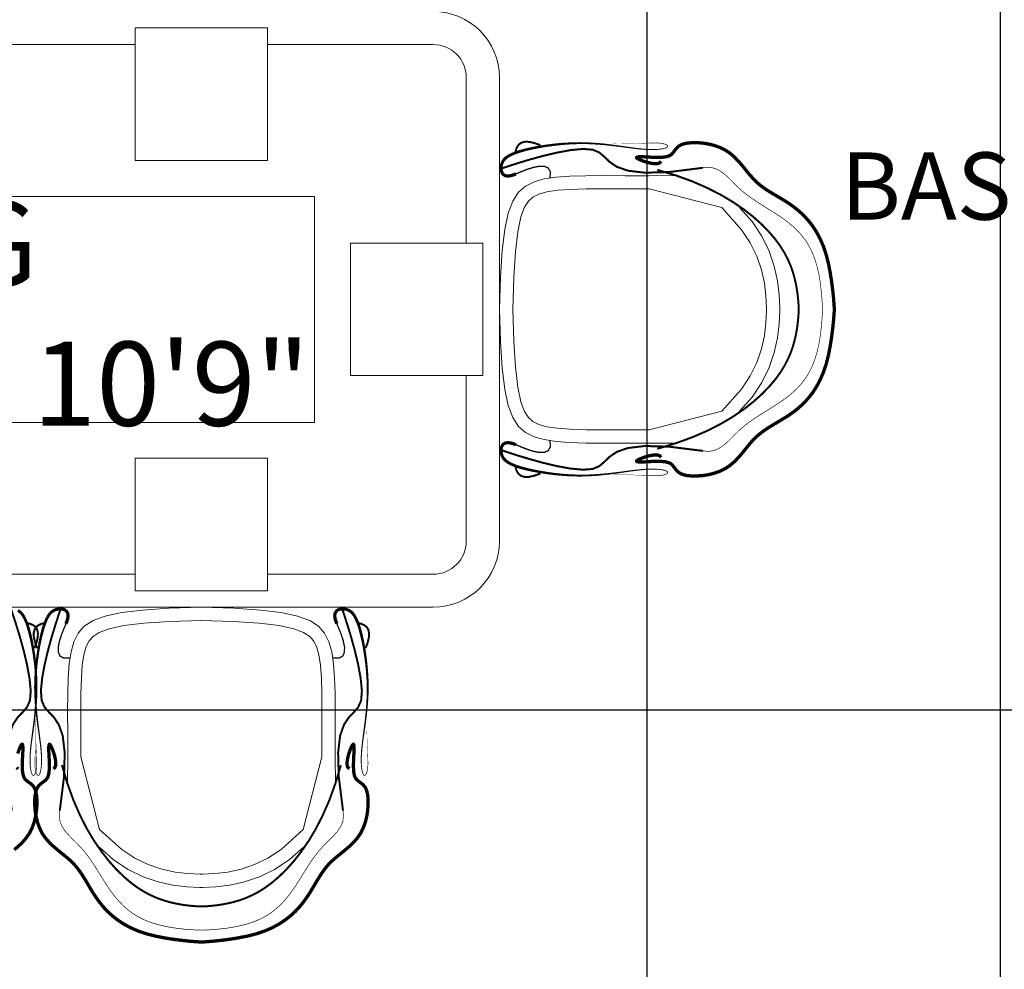
# Model space of a CAD drawing. Units: inches. Extents: x 870 to 1431, y 383 to 1070.
# Tile 6 of 9: x 1171 to 1230, y 661 to 718. Entities that reach past the tile are written whole.
import ezdxf

# ---------------------------------------------------------------- set-up
doc = ezdxf.new("R2010")
doc.units = ezdxf.units.IN
doc.header["$MEASUREMENT"] = 0
for name, color, linetype, lineweight in [('A-ANNO-DIMS', 2, 'Continuous', 18), ('A-AREA-IDEN', 7, 'Continuous', 25), ('A-FURN', 8, 'Continuous', 18)]:
    doc.layers.add(name, color=color, linetype=linetype, lineweight=lineweight)
doc.styles.get("Standard").update_dxf_attribs({"font": 'arial.ttf'})
doc.dimstyles.get("Standard").update_dxf_attribs({"dimtxt": 4, "dimasz": 0.18, "dimexe": 0.18, "dimexo": 0.0625, "dimgap": 0.09, "dimtad": 0, "dimtih": 1, "dimtoh": 1, "dimdec": 0, "dimrnd": 6, "dimzin": 0, "dimdsep": 46, "dimlunit": 3, "dimtxsty": 'Standard', "dimcen": 0.09, "dimadec": 0, "dimazin": 0, "dimtfac": 1, "dimtdec": 0, "dimtofl": 0, "dimtmove": 0, "dimatfit": 3, "dimfxl": 1, "dimtolj": 1, "dimtzin": 0, "dimarcsym": 0})

# ---------------------------------------------------------------- blocks, each defined once
blk = doc.blocks.new('ОГ53_на8персон_стол1900х900')
for p, q in [((400, 254.3), (400, 54.3)), ((600, 254.3), (400, 254.3)), ((600, 54.3), (600, 254.3)), ((100, 229.3), (400, 229.3)), ((600, 229.3), (850, 229.3)), ((900, 179.3), (900, -70.7)), ((950, 179.3), (950, -520.7)), ((400, 54.3), (600, 54.3)), ((670.7, 0), (-670.7, 0)), ((670.7, -341.4), (670.7, 0)), ((725, -270.7), (725, -70.7)), ((725, -70.7), (925, -70.7)), ((925, -70.7), (925, -270.7)), ((925, -270.7), (725, -270.7)), ((900, -270.7), (900, -520.7)), ((-670.7, -341.4), (670.7, -341.4)), ((400, -595.7), (400, -395.7)), ((400, -395.7), (600, -395.7)), ((600, -395.7), (600, -595.7)), ((400, -570.7), (100, -570.7)), ((850, -570.7), (600, -570.7)), ((600, -595.7), (400, -595.7)), ((850, -620.7), (-850, -620.7))]:
    blk.add_line(p, q)
for points in [[(974.9, 33.8, 5, 4.91, 0), (968.1, 31.4, 4.91, 4.84, 0), (962.8, 30.6, 4.84, 4.78, 0), (958.7, 31.2, 4.78, 4.74, 0), (955.8, 33, 4.74, 4.7, 0), (953.9, 35.6, 4.7, 4.65, 0), (952.9, 38.8, 4.65, 4.61, 0), (952.5, 42.3, 4.61, 4.56, 0), (952.8, 45.8, 4.56, 4.52, 0), (953.5, 49.1, 4.52, 4.47, 0), (954.8, 52.2, 4.47, 4.43, 0), (956.7, 55.2, 4.43, 4.38, 0), (959.5, 58, 4.38, 4.32, 0), (963.2, 60.6, 4.32, 4.25, 0), (967.9, 63.2, 4.25, 4.17, 0), (973.8, 65.6, 4.17, 4.07, 0), (981, 68, 4.07, 3.95, 0), (989.6, 70.4, 3.95, 3.82, 0), (999.3, 72.6, 3.82, 3.68, 0), (1010.1, 74.7, 3.68, 3.53, 0), (1021.6, 76.5, 3.53, 3.37, 0), (1033.7, 78.1, 3.37, 3.21, 0), (1046.2, 79.3, 3.21, 3.05, 0), (1058.8, 80.1, 3.05, 2.88, 0), (1071.4, 80.4, 2.88, 2.72, 0), (1083.8, 80.2, 2.72, 2.57, 0), (1095.8, 79.5, 2.57, 2.41, 0), (1107.4, 78.6, 2.41, 2.27, 0), (1118.5, 77.3, 2.27, 2.13, 0), (1129, 76, 2.13, 2, 0), (1138.9, 74.6, 2, 1.88, 0), (1148, 73.4, 1.88, 1.78, 0), (1156.3, 72.3, 1.78, 1.68, 0), (1163.7, 71.5, 1.68, 1.59, 0), (1170.3, 71, 1.59, 1.52, 0), (1176.1, 70.7, 1.52, 1.45, 0), (1181.2, 70.7, 1.45, 1.4, 0), (1185.6, 70.7, 1.4, 1.35, 0), (1189.4, 71, 1.35, 1.3, 0), (1192.6, 71.3, 1.3, 1.27, 0), (1195.3, 71.7, 1.27, 1.24, 0), (1197.6, 72.1, 1.24, 1.21, 0), (1199.5, 72.6, 1.21, 1.19, 0), (1201, 73.1, 1.19, 1.18, 0), (1202.2, 73.6, 1.18, 1.16, 0), (1203, 74.1, 1.16, 1.15, 0), (1203.6, 74.6, 1.15, 1.14, 0), (1203.9, 75.1, 1.14, 1.14, 0), (1204, 75.6, 1.14, 1.13, 0), (1203.9, 76.2, 1.13, 1.12, 0), (1203.6, 76.6, 1.12, 1.12, 0), (1203.2, 77.1, 1.12, 1.11, 0), (1202.6, 77.6, 1.11, 1.09, 0), (1201.8, 78, 1.09, 1.08, 0), (1200.9, 78.4, 1.08, 1.07, 0), (1199.8, 78.9, 1.07, 1.05, 0), (1198.6, 79.2, 1.05, 1.03, 0), (1197.2, 79.6, 1.03, 1.01, 0), (1195.6, 79.9, 1.01, 0.986, 0), (1193.8, 80.2, 0.986, 0.959, 0), (1191.7, 80.4, 0.959, 0.926, 0), (1189.2, 80.6, 0.926, 0.889, 0), (1186.3, 80.7, 0.889, 0.846, 0), (1183, 80.7, 0.846, 0.796, 0), (1179.1, 80.6, 0.796, 0.738, 0), (1174.7, 80.4, 0.738, 0.672, 0), (1169.6, 80.2, 0.672, 0.595, 0), (1163.7, 79.9, 0.595, 0.506, 0), (1156.8, 79.6, 0.506, 0.404, 0), (1148.9, 79.4, 0.404, 0.286, 0), (1139.9, 79.2, 0.286, 0.152, 0), (1129.5, 79.2, 0.152, 0, 0), (1117.8, 79.4, 0, 0, 0)], [(974.9, -375.1, 5, 4.91, 0), (968.1, -372.7, 4.91, 4.84, 0), (962.8, -372, 4.84, 4.78, 0), (958.7, -372.6, 4.78, 4.74, 0), (955.8, -374.3, 4.74, 4.7, 0), (953.9, -376.9, 4.7, 4.65, 0), (952.9, -380.1, 4.65, 4.61, 0), (952.5, -383.6, 4.61, 4.56, 0), (952.8, -387.1, 4.56, 4.52, 0), (953.5, -390.5, 4.52, 4.47, 0), (954.8, -393.6, 4.47, 4.43, 0), (956.7, -396.6, 4.43, 4.38, 0), (959.5, -399.3, 4.38, 4.32, 0), (963.2, -402, 4.32, 4.25, 0), (967.9, -404.5, 4.25, 4.17, 0), (973.8, -407, 4.17, 4.07, 0), (981, -409.4, 4.07, 3.95, 0), (989.6, -411.7, 3.95, 3.82, 0), (999.3, -414, 3.82, 3.68, 0), (1010.1, -416, 3.68, 3.53, 0), (1021.6, -417.9, 3.53, 3.37, 0), (1033.7, -419.5, 3.37, 3.21, 0), (1046.2, -420.7, 3.21, 3.05, 0), (1058.8, -421.5, 3.05, 2.88, 0), (1071.4, -421.8, 2.88, 2.72, 0), (1083.8, -421.6, 2.72, 2.57, 0), (1095.8, -420.9, 2.57, 2.41, 0), (1107.4, -419.9, 2.41, 2.27, 0), (1118.5, -418.7, 2.27, 2.13, 0), (1129, -417.4, 2.13, 2, 0), (1138.9, -416, 2, 1.88, 0), (1148, -414.7, 1.88, 1.78, 0), (1156.3, -413.7, 1.78, 1.68, 0), (1163.7, -412.9, 1.68, 1.59, 0), (1170.3, -412.4, 1.59, 1.52, 0), (1176.1, -412.1, 1.52, 1.45, 0), (1181.2, -412, 1.45, 1.4, 0), (1185.6, -412.1, 1.4, 1.35, 0), (1189.4, -412.3, 1.35, 1.3, 0), (1192.6, -412.7, 1.3, 1.27, 0), (1195.3, -413, 1.27, 1.24, 0), (1197.6, -413.5, 1.24, 1.21, 0), (1199.5, -413.9, 1.21, 1.19, 0), (1201, -414.4, 1.19, 1.18, 0), (1202.2, -414.9, 1.18, 1.16, 0), (1203, -415.4, 1.16, 1.15, 0), (1203.6, -416, 1.15, 1.14, 0), (1203.9, -416.5, 1.14, 1.14, 0), (1204, -417, 1.14, 1.13, 0), (1203.9, -417.5, 1.13, 1.12, 0), (1203.6, -418, 1.12, 1.12, 0), (1203.2, -418.5, 1.12, 1.11, 0), (1202.6, -418.9, 1.11, 1.09, 0), (1201.8, -419.4, 1.09, 1.08, 0), (1200.9, -419.8, 1.08, 1.07, 0), (1199.8, -420.2, 1.07, 1.05, 0), (1198.6, -420.6, 1.05, 1.03, 0), (1197.2, -421, 1.03, 1.01, 0), (1195.6, -421.3, 1.01, 0.986, 0), (1193.8, -421.6, 0.986, 0.959, 0), (1191.7, -421.8, 0.959, 0.926, 0), (1189.2, -422, 0.926, 0.889, 0), (1186.3, -422, 0.889, 0.846, 0), (1183, -422, 0.846, 0.796, 0), (1179.1, -422, 0.796, 0.738, 0), (1174.7, -421.8, 0.738, 0.672, 0), (1169.6, -421.5, 0.672, 0.595, 0), (1163.7, -421.2, 0.595, 0.506, 0), (1156.8, -421, 0.506, 0.404, 0), (1148.9, -420.7, 0.404, 0.286, 0), (1139.9, -420.6, 0.286, 0.152, 0), (1129.5, -420.6, 0.152, 0, 0), (1117.8, -420.7, 0, 0, 0)], [(222.9, -625.5, 4.47, 4.43, 0), (225.9, -627.4, 4.43, 4.38, 0), (228.7, -630.2, 4.38, 4.32, 0), (231.3, -633.9, 4.32, 4.25, 0), (233.8, -638.6, 4.25, 4.17, 0), (236.3, -644.5, 4.17, 4.07, 0), (238.7, -651.7, 4.07, 3.95, 0), (241, -660.3, 3.95, 3.82, 0), (243.3, -670, 3.82, 3.68, 0), (245.4, -680.8, 3.68, 3.53, 0), (247.2, -692.3, 3.53, 3.37, 0), (248.8, -704.4, 3.37, 3.21, 0), (250, -716.9, 3.21, 3.05, 0), (250.8, -729.5, 3.05, 2.88, 0), (251.1, -742.1, 2.88, 2.72, 0), (250.9, -754.5, 2.72, 2.57, 0), (250.2, -766.5, 2.57, 2.41, 0), (249.2, -778.1, 2.41, 2.27, 0), (248, -789.2, 2.27, 2.13, 0), (246.7, -799.7, 2.13, 2, 0), (245.3, -809.6, 2, 1.88, 0), (244.1, -818.7, 1.88, 1.78, 0), (243, -827, 1.78, 1.68, 0), (242.2, -834.4, 1.68, 1.59, 0), (241.7, -841, 1.59, 1.52, 0), (241.4, -846.8, 1.52, 1.45, 0), (241.3, -851.9, 1.45, 1.4, 0), (241.4, -856.3, 1.4, 1.35, 0), (241.6, -860.1, 1.35, 1.3, 0), (242, -863.3, 1.3, 1.27, 0), (242.4, -866, 1.27, 1.24, 0), (242.8, -868.3, 1.24, 1.21, 0), (243.3, -870.2, 1.21, 1.19, 0), (243.8, -871.7, 1.19, 1.18, 0), (244.3, -872.9, 1.18, 1.16, 0), (244.8, -873.7, 1.16, 1.15, 0), (245.3, -874.3, 1.15, 1.14, 0), (245.8, -874.6, 1.14, 1.14, 0), (246.3, -874.7, 1.14, 1.13, 0), (246.8, -874.6, 1.13, 1.12, 0), (247.3, -874.3, 1.12, 1.12, 0), (247.8, -873.9, 1.12, 1.11, 0), (248.3, -873.3, 1.11, 1.09, 0), (248.7, -872.5, 1.09, 1.08, 0), (249.1, -871.6, 1.08, 1.07, 0), (249.5, -870.5, 1.07, 1.05, 0), (249.9, -869.2, 1.05, 1.03, 0), (250.3, -867.9, 1.03, 1.01, 0), (250.6, -866.3, 1.01, 0.986, 0), (250.9, -864.5, 0.986, 0.959, 0), (251.1, -862.4, 0.959, 0.926, 0), (251.3, -859.9, 0.926, 0.889, 0), (251.4, -857, 0.889, 0.846, 0), (251.4, -853.7, 0.846, 0.796, 0), (251.3, -849.8, 0.796, 0.738, 0), (251.1, -845.4, 0.738, 0.672, 0), (250.8, -840.3, 0.672, 0.595, 0), (250.6, -834.3, 0.595, 0.506, 0), (250.3, -827.5, 0.506, 0.404, 0), (250.1, -819.6, 0.404, 0.286, 0), (249.9, -810.5, 0.286, 0.152, 0), (249.9, -800.2, 0.152, 0, 0), (250, -788.5, 0, 0, 0)], [(295.5, -645.6, 5, 4.91, 0), (298, -638.8, 4.91, 4.84, 0), (298.7, -633.5, 4.84, 4.78, 0), (298.1, -629.4, 4.78, 4.74, 0), (296.3, -626.5, 4.74, 4.7, 0), (293.7, -624.6, 4.7, 4.65, 0), (290.6, -623.5, 4.65, 4.61, 0), (287.1, -623.2, 4.61, 4.56, 0), (283.5, -623.5, 4.56, 4.52, 0), (280.2, -624.2, 4.52, 4.47, 0), (277.1, -625.5, 4.47, 4.43, 0), (274.1, -627.4, 4.43, 4.38, 0), (271.3, -630.2, 4.38, 4.32, 0), (268.7, -633.9, 4.32, 4.25, 0), (266.2, -638.6, 4.25, 4.17, 0), (263.7, -644.5, 4.17, 4.07, 0), (261.3, -651.7, 4.07, 3.95, 0), (259, -660.3, 3.95, 3.82, 0), (256.7, -670, 3.82, 3.68, 0), (254.6, -680.8, 3.68, 3.53, 0), (252.8, -692.3, 3.53, 3.37, 0), (251.2, -704.4, 3.37, 3.21, 0), (250, -716.9, 3.21, 3.05, 0), (249.2, -729.5, 3.05, 2.88, 0), (248.9, -742.1, 2.88, 2.72, 0), (249.1, -754.5, 2.72, 2.57, 0), (249.8, -766.5, 2.57, 2.41, 0), (250.8, -778.1, 2.41, 2.27, 0), (252, -789.2, 2.27, 2.13, 0), (253.3, -799.7, 2.13, 2, 0), (254.7, -809.6, 2, 1.88, 0), (255.9, -818.7, 1.88, 1.78, 0), (257, -827, 1.78, 1.68, 0), (257.8, -834.4, 1.68, 1.59, 0), (258.3, -841, 1.59, 1.52, 0), (258.6, -846.8, 1.52, 1.45, 0), (258.7, -851.9, 1.45, 1.4, 0), (258.6, -856.3, 1.4, 1.35, 0), (258.4, -860.1, 1.35, 1.3, 0), (258, -863.3, 1.3, 1.27, 0), (257.6, -866, 1.27, 1.24, 0), (257.2, -868.3, 1.24, 1.21, 0), (256.7, -870.2, 1.21, 1.19, 0), (256.2, -871.7, 1.19, 1.18, 0), (255.7, -872.9, 1.18, 1.16, 0), (255.2, -873.7, 1.16, 1.15, 0), (254.7, -874.3, 1.15, 1.14, 0), (254.2, -874.6, 1.14, 1.14, 0), (253.7, -874.7, 1.14, 1.13, 0), (253.2, -874.6, 1.13, 1.12, 0), (252.7, -874.3, 1.12, 1.12, 0), (252.2, -873.9, 1.12, 1.11, 0), (251.7, -873.3, 1.11, 1.09, 0), (251.3, -872.5, 1.09, 1.08, 0), (250.9, -871.6, 1.08, 1.07, 0), (250.5, -870.5, 1.07, 1.05, 0), (250.1, -869.2, 1.05, 1.03, 0), (249.7, -867.9, 1.03, 1.01, 0), (249.4, -866.3, 1.01, 0.986, 0), (249.1, -864.5, 0.986, 0.959, 0), (248.9, -862.4, 0.959, 0.926, 0), (248.7, -859.9, 0.926, 0.889, 0), (248.6, -857, 0.889, 0.846, 0), (248.6, -853.7, 0.846, 0.796, 0), (248.7, -849.8, 0.796, 0.738, 0), (248.9, -845.4, 0.738, 0.672, 0), (249.2, -840.3, 0.672, 0.595, 0), (249.4, -834.3, 0.595, 0.506, 0), (249.7, -827.5, 0.506, 0.404, 0), (249.9, -819.6, 0.404, 0.286, 0), (250.1, -810.5, 0.286, 0.152, 0), (250.1, -800.2, 0.152, 0, 0), (250, -788.5, 0, 0, 0)], [(704.5, -645.6, 5, 4.91, 0), (702, -638.8, 4.91, 4.84, 0), (701.3, -633.5, 4.84, 4.78, 0), (701.9, -629.4, 4.78, 4.74, 0), (703.7, -626.5, 4.74, 4.7, 0), (706.3, -624.6, 4.7, 4.65, 0), (709.4, -623.5, 4.65, 4.61, 0), (712.9, -623.2, 4.61, 4.56, 0), (716.5, -623.5, 4.56, 4.52, 0), (719.8, -624.2, 4.52, 4.47, 0), (722.9, -625.5, 4.47, 4.43, 0), (725.9, -627.4, 4.43, 4.38, 0), (728.7, -630.2, 4.38, 4.32, 0), (731.3, -633.9, 4.32, 4.25, 0), (733.8, -638.6, 4.25, 4.17, 0), (736.3, -644.5, 4.17, 4.07, 0), (738.7, -651.7, 4.07, 3.95, 0), (741, -660.3, 3.95, 3.82, 0), (743.3, -670, 3.82, 3.68, 0), (745.4, -680.8, 3.68, 3.53, 0), (747.2, -692.3, 3.53, 3.37, 0), (748.8, -704.4, 3.37, 3.21, 0), (750, -716.9, 3.21, 3.05, 0), (750.8, -729.5, 3.05, 2.88, 0), (751.1, -742.1, 2.88, 2.72, 0), (750.9, -754.5, 2.72, 2.57, 0), (750.2, -766.5, 2.57, 2.41, 0), (749.2, -778.1, 2.41, 2.27, 0), (748, -789.2, 2.27, 2.13, 0), (746.7, -799.7, 2.13, 2, 0), (745.3, -809.6, 2, 1.88, 0), (744.1, -818.7, 1.88, 1.78, 0), (743, -827, 1.78, 1.68, 0), (742.2, -834.4, 1.68, 1.59, 0), (741.7, -841, 1.59, 1.52, 0), (741.4, -846.8, 1.52, 1.45, 0), (741.3, -851.9, 1.45, 1.4, 0), (741.4, -856.3, 1.4, 1.35, 0), (741.6, -860.1, 1.35, 1.3, 0), (742, -863.3, 1.3, 1.27, 0), (742.4, -866, 1.27, 1.24, 0), (742.8, -868.3, 1.24, 1.21, 0), (743.3, -870.2, 1.21, 1.19, 0), (743.8, -871.7, 1.19, 1.18, 0), (744.3, -872.9, 1.18, 1.16, 0), (744.8, -873.7, 1.16, 1.15, 0), (745.3, -874.3, 1.15, 1.14, 0), (745.8, -874.6, 1.14, 1.14, 0), (746.3, -874.7, 1.14, 1.13, 0), (746.8, -874.6, 1.13, 1.12, 0), (747.3, -874.3, 1.12, 1.12, 0), (747.8, -873.9, 1.12, 1.11, 0), (748.3, -873.3, 1.11, 1.09, 0), (748.7, -872.5, 1.09, 1.08, 0), (749.1, -871.6, 1.08, 1.07, 0), (749.5, -870.5, 1.07, 1.05, 0), (749.9, -869.2, 1.05, 1.03, 0), (750.3, -867.9, 1.03, 1.01, 0), (750.6, -866.3, 1.01, 0.986, 0), (750.9, -864.5, 0.986, 0.959, 0), (751.1, -862.4, 0.959, 0.926, 0), (751.3, -859.9, 0.926, 0.889, 0), (751.4, -857, 0.889, 0.846, 0), (751.4, -853.7, 0.846, 0.796, 0), (751.3, -849.8, 0.796, 0.738, 0), (751.1, -845.4, 0.738, 0.672, 0), (750.8, -840.3, 0.672, 0.595, 0), (750.6, -834.3, 0.595, 0.506, 0), (750.3, -827.5, 0.506, 0.404, 0), (750.1, -819.6, 0.404, 0.286, 0), (749.9, -810.5, 0.286, 0.152, 0), (749.9, -800.2, 0.152, 0, 0), (750, -788.5, 0, 0, 0)]]:
    blk.add_lwpolyline(points, format="xyseb")
for points, const_width in [([(1011.7, 77.3), (1002.5, 80.6), (994.8, 82.3), (988.5, 82.4), (983.5, 81.2), (979.7, 78.7), (976.9, 75.1), (975, 70.5), (973.8, 65)], 3), ([(1194.1, 52.8), (1192.1, 50.6), (1188.9, 49.4), (1184.9, 49.2), (1180.3, 49.7), (1175.5, 50.7), (1170.8, 52), (1166.4, 53.5), (1162.7, 55), (1159.9, 56.3), (1158, 57.4), (1157.1, 58.2), (1157.1, 58.9), (1158, 59.4), (1159.8, 59.7), (1162.5, 59.9), (1166.1, 59.8), (1170.5, 59.6), (1175.5, 59.3), (1181, 59), (1186.6, 58.9), (1192.2, 58.9), (1197.5, 59.2), (1202.2, 59.9), (1206.2, 61.1), (1209.2, 62.9), (1211.5, 65), (1213.4, 67.5), (1215.3, 70.1), (1217.4, 72.7), (1219.9, 75.2), (1223.4, 77.4), (1227.9, 79.2), (1233.8, 80.4), (1240.9, 81.1), (1248.8, 81.1), (1257.3, 80.4), (1266.1, 78.9), (1274.9, 76.7), (1283.4, 73.6), (1291.3, 69.7), (1298.4, 64.9), (1304.8, 59.3), (1310.7, 53.2), (1316.3, 46.8), (1321.6, 40.2), (1326.9, 33.7), (1332.4, 27.4), (1338.1, 21.5), (1344.4, 16.2), (1351, 11.4), (1358, 6.9), (1365.2, 2.5), (1372.6, -1.8), (1380.1, -6.3), (1387.6, -11.1), (1395, -16.4), (1402.3, -22.3), (1409.4, -29), (1416.2, -36.3), (1422.7, -44.6), (1428.7, -53.8), (1434.1, -64), (1439, -75.2), (1443.2, -87.7), (1446.7, -101.2), (1449.4, -115.3), (1451.6, -129.2), (1453.2, -142.1), (1454.4, -153.5), (1455.1, -162.5), (1455.5, -168.5), (1455.7, -170.7)], 5), ([(1257.2, 43.1), (1206.2, 36.7), (1169.4, 35.7), (1144.1, 38.7), (1127.3, 44.6), (1116.4, 51.9), (1108.5, 59.6), (1100.8, 66.2), (1090.7, 70.5), (1076, 71.6), (1057.4, 69.8), (1036.6, 66), (1015.2, 60.9), (994.5, 55.2), (976.1, 49.6), (961.6, 44.9), (952.6, 41.8)], 3), ([(974.9, 33.8), (982.7, 37.2), (991.6, 40.7), (1001, 43.6), (1010, 45.4), (1017.8, 45.4), (1023.6, 42.8), (1026.8, 37.1), (1026.4, 27.6)], 2), ([(1188.3, 40), (1216.1, 31.7), (1241.4, 22.5), (1264.2, 12.5), (1284.8, 2), (1303.1, -8.9), (1319.4, -20.1), (1333.7, -31.3), (1346.1, -42.5), (1356.8, -53.5), (1366, -64.2), (1373.7, -74.7), (1380.1, -84.9), (1385.3, -94.9), (1389.6, -104.7), (1393, -114.3), (1395.6, -123.7), (1397.7, -132.7), (1399.2, -141.4), (1400.3, -149.3), (1401, -156.4), (1401.5, -162.3), (1401.7, -166.8), (1401.8, -169.6), (1401.8, -170.7)], 3), ([(1257.2, 43.1), (1265.9, 43.9), (1273.6, 42.7), (1280.7, 39.8), (1287.3, 35.6), (1293.5, 30.4), (1299.4, 24.7), (1305.3, 18.6), (1311.3, 12.7), (1317.5, 7.2), (1323.9, 2.1), (1330.6, -2.8), (1337.4, -7.4), (1344.3, -11.8), (1351.4, -16.3), (1358.5, -20.7), (1365.7, -25.2), (1372.9, -29.9), (1380, -34.9), (1387, -40.2), (1393.8, -45.9), (1400.3, -52.2), (1406.4, -59), (1412.1, -66.5), (1417.3, -74.8), (1421.9, -83.9), (1425.9, -94), (1429.3, -105.1), (1432.2, -117.4), (1434.5, -130.9), (1436.2, -145.8), (1437.4, -162.1), (1437.8, -170.7)], 1), ([(1194.1, -394.1), (1192.1, -391.9), (1188.9, -390.8), (1184.9, -390.6), (1180.3, -391.1), (1175.5, -392), (1170.8, -393.4), (1166.4, -394.9), (1162.7, -396.3), (1159.9, -397.6), (1158, -398.7), (1157.1, -399.6), (1157.1, -400.3), (1158, -400.8), (1159.8, -401.1), (1162.5, -401.2), (1166.1, -401.2), (1170.5, -401), (1175.5, -400.7), (1181, -400.4), (1186.6, -400.2), (1192.2, -400.3), (1197.5, -400.6), (1202.2, -401.3), (1206.2, -402.5), (1209.2, -404.2), (1211.5, -406.4), (1213.4, -408.8), (1215.3, -411.4), (1217.4, -414.1), (1219.9, -416.5), (1223.4, -418.7), (1227.9, -420.5), (1233.8, -421.8), (1240.9, -422.4), (1248.8, -422.4), (1257.3, -421.7), (1266.1, -420.3), (1274.9, -418), (1283.4, -415), (1291.3, -411), (1298.4, -406.2), (1304.8, -400.7), (1310.7, -394.6), (1316.3, -388.1), (1321.6, -381.6), (1326.9, -375), (1332.4, -368.7), (1338.1, -362.9), (1344.4, -357.6), (1351, -352.8), (1358, -348.2), (1365.2, -343.9), (1372.6, -339.5), (1380.1, -335), (1387.6, -330.2), (1395, -324.9), (1402.3, -319), (1409.4, -312.4), (1416.2, -305), (1422.7, -296.8), (1428.7, -287.6), (1434.1, -277.4), (1439, -266.1), (1443.2, -253.7), (1446.7, -240.1), (1449.4, -226.1), (1451.6, -212.2), (1453.2, -199.2), (1454.4, -187.9), (1455.1, -178.9), (1455.5, -172.9), (1455.7, -170.7)], 5), ([(1188.3, -381.3), (1216.1, -373), (1241.4, -363.8), (1264.2, -353.9), (1284.8, -343.4), (1303.1, -332.5), (1319.4, -321.3), (1333.7, -310), (1346.1, -298.9), (1356.8, -287.9), (1366, -277.2), (1373.7, -266.7), (1380.1, -256.4), (1385.3, -246.4), (1389.6, -236.6), (1393, -227), (1395.6, -217.7), (1397.7, -208.6), (1399.2, -200), (1400.3, -192), (1401, -185), (1401.5, -179.1), (1401.7, -174.6), (1401.8, -171.7), (1401.8, -170.7)], 3), ([(1257.2, -384.5), (1265.9, -385.3), (1273.6, -384), (1280.7, -381.1), (1287.3, -376.9), (1293.5, -371.8), (1299.4, -366), (1305.3, -360), (1311.3, -354.1), (1317.5, -348.6), (1323.9, -343.4), (1330.6, -338.6), (1337.4, -334), (1344.3, -329.5), (1351.4, -325.1), (1358.5, -320.7), (1365.7, -316.1), (1372.9, -311.4), (1380, -306.5), (1387, -301.2), (1393.8, -295.4), (1400.3, -289.2), (1406.4, -282.3), (1412.1, -274.8), (1417.3, -266.5), (1421.9, -257.4), (1425.9, -247.3), (1429.3, -236.2), (1432.2, -224), (1434.5, -210.5), (1436.2, -195.6), (1437.4, -179.3), (1437.8, -170.7)], 1), ([(974.9, -375.1), (982.7, -378.5), (991.6, -382), (1001, -385), (1010, -386.8), (1017.8, -386.7), (1023.6, -384.2), (1026.8, -378.4), (1026.4, -368.9)], 2), ([(1257.2, -384.5), (1206.2, -378.1), (1169.4, -377.1), (1144.1, -380.1), (1127.3, -385.9), (1116.4, -393.3), (1108.5, -400.9), (1100.8, -407.5), (1090.7, -411.8), (1076, -412.9), (1057.4, -411.2), (1036.6, -407.4), (1015.2, -402.3), (994.5, -396.5), (976.1, -391), (961.6, -386.3), (952.6, -383.2)], 3), ([(1011.7, -418.7), (1002.5, -422), (994.8, -423.7), (988.5, -423.8), (983.5, -422.6), (979.7, -420.1), (976.9, -416.5), (975, -411.9), (973.8, -406.4)], 3), ([(213.8, -927.9), (207.4, -876.9), (206.4, -840.1), (209.4, -814.7), (215.3, -798), (222.6, -787), (230.2, -779.2), (236.8, -771.5), (241.2, -761.4), (242.3, -746.6), (240.5, -728.1), (236.7, -707.3), (231.6, -685.8), (225.9, -665.1), (220.3, -646.8), (215.6, -632.3), (212.5, -623.2)], 3), ([(286.2, -927.9), (292.6, -876.9), (293.6, -840.1), (290.6, -814.7), (284.7, -798), (277.4, -787), (269.8, -779.2), (263.2, -771.5), (258.8, -761.4), (257.7, -746.6), (259.5, -728.1), (263.3, -707.3), (268.4, -685.8), (274.1, -665.1), (279.7, -646.8), (284.4, -632.3), (287.5, -623.2)], 3), ([(713.8, -927.9), (707.4, -876.9), (706.4, -840.1), (709.4, -814.7), (715.3, -798), (722.6, -787), (730.2, -779.2), (736.8, -771.5), (741.2, -761.4), (742.3, -746.6), (740.5, -728.1), (736.7, -707.3), (731.6, -685.8), (725.9, -665.1), (720.3, -646.8), (715.6, -632.3), (712.5, -623.2)], 3), ([(248, -682.4), (251.3, -673.2), (253, -665.5), (253.1, -659.2), (251.9, -654.2), (249.4, -650.4), (245.8, -647.6), (241.2, -645.6), (235.7, -644.5)], 3), ([(252, -682.4), (248.7, -673.2), (247, -665.5), (246.9, -659.2), (248.1, -654.2), (250.6, -650.4), (254.2, -647.6), (258.8, -645.6), (264.3, -644.5)], 3), ([(295.5, -645.6), (292.2, -653.4), (288.7, -662.3), (285.7, -671.7), (283.9, -680.7), (284, -688.5), (286.5, -694.3), (292.2, -697.5), (301.8, -697.1)], 2), ([(704.5, -645.6), (707.8, -653.4), (711.3, -662.3), (714.3, -671.7), (716.1, -680.7), (716, -688.5), (713.5, -694.3), (707.8, -697.5), (698.2, -697.1)], 2), ([(748, -682.4), (751.3, -673.2), (753, -665.5), (753.1, -659.2), (751.9, -654.2), (749.4, -650.4), (745.8, -647.6), (741.2, -645.6), (735.7, -644.5)], 3), ([(223.4, -864.8), (221.2, -862.7)], 5), ([(222.7, -841.5), (224.2, -837.1), (225.7, -833.4), (227, -830.6), (228, -828.7), (228.9, -827.8), (229.6, -827.7), (230.1, -828.6), (230.4, -830.5), (230.6, -833.2), (230.5, -836.7), (230.3, -841.2), (230, -846.2), (229.7, -851.7), (229.6, -857.3), (229.6, -862.9), (229.9, -868.2), (230.6, -872.9), (231.8, -876.8), (233.5, -879.9), (235.7, -882.2), (238.2, -884.1), (240.8, -886), (243.4, -888), (245.9, -890.6), (248.1, -894), (249.8, -898.6), (251.1, -904.5), (251.7, -911.6), (251.7, -919.5), (251, -928), (249.6, -936.8), (247.4, -945.6), (244.3, -954.1), (240.4, -962), (235.5, -969.1), (230, -975.5), (223.9, -981.4), (217.5, -986.9)], 5), ([(276.6, -864.8), (278.8, -862.7), (279.9, -859.6), (280.1, -855.5), (279.6, -851), (278.6, -846.2), (277.3, -841.5), (275.8, -837.1), (274.3, -833.4), (273, -830.6), (272, -828.7), (271.1, -827.8), (270.4, -827.7), (269.9, -828.6), (269.6, -830.5), (269.4, -833.2), (269.5, -836.7), (269.7, -841.2), (270, -846.2), (270.3, -851.7), (270.4, -857.3), (270.4, -862.9), (270.1, -868.2), (269.4, -872.9), (268.2, -876.8), (266.5, -879.9), (264.3, -882.2), (261.8, -884.1), (259.2, -886), (256.6, -888), (254.1, -890.6), (251.9, -894), (250.2, -898.6), (248.9, -904.5), (248.3, -911.6), (248.3, -919.5), (249, -928), (250.4, -936.8), (252.6, -945.6), (255.7, -954.1), (259.6, -962), (264.5, -969.1), (270, -975.5), (276.1, -981.4), (282.5, -986.9), (289.1, -992.3), (295.7, -997.6), (301.9, -1003), (307.8, -1008.8), (313.1, -1015.1), (317.9, -1021.7), (322.4, -1028.7), (326.8, -1035.9), (331.1, -1043.3), (335.6, -1050.8), (340.5, -1058.3), (345.8, -1065.7), (351.7, -1073), (358.3, -1080.1), (365.7, -1086.9), (373.9, -1093.3), (383.1, -1099.3), (393.3, -1104.8), (404.6, -1109.7), (417, -1113.9), (430.5, -1117.3), (444.6, -1120.1), (458.5, -1122.3), (471.4, -1123.9), (482.8, -1125.1), (491.8, -1125.8), (497.8, -1126.2), (500, -1126.3)], 5), ([(723.4, -864.8), (721.2, -862.7), (720.1, -859.6), (719.9, -855.5), (720.4, -851), (721.4, -846.2), (722.7, -841.5), (724.2, -837.1), (725.7, -833.4), (727, -830.6), (728, -828.7), (728.9, -827.8), (729.6, -827.7), (730.1, -828.6), (730.4, -830.5), (730.6, -833.2), (730.5, -836.7), (730.3, -841.2), (730, -846.2), (729.7, -851.7), (729.6, -857.3), (729.6, -862.9), (729.9, -868.2), (730.6, -872.9), (731.8, -876.8), (733.5, -879.9), (735.7, -882.2), (738.2, -884.1), (740.8, -886), (743.4, -888), (745.9, -890.6), (748.1, -894), (749.8, -898.6), (751.1, -904.5), (751.7, -911.6), (751.7, -919.5), (751, -928), (749.6, -936.8), (747.4, -945.6), (744.3, -954.1), (740.4, -962), (735.5, -969.1), (730, -975.5), (723.9, -981.4), (717.5, -986.9), (710.9, -992.3), (704.3, -997.6), (698.1, -1003), (692.2, -1008.8), (686.9, -1015.1), (682.1, -1021.7), (677.6, -1028.7), (673.2, -1035.9), (668.9, -1043.3), (664.4, -1050.8), (659.5, -1058.3), (654.2, -1065.7), (648.3, -1073), (641.7, -1080.1), (634.3, -1086.9), (626.1, -1093.3), (616.9, -1099.3), (606.7, -1104.8), (595.4, -1109.7), (583, -1113.9), (569.5, -1117.3), (555.4, -1120.1), (541.5, -1122.3), (528.6, -1123.9), (517.2, -1125.1), (508.2, -1125.8), (502.2, -1126.2), (500, -1126.3)], 5), ([(289.4, -859), (297.7, -886.8), (306.8, -912.1), (316.8, -934.9), (327.3, -955.5), (338.2, -973.8), (349.4, -990), (360.6, -1004.3), (371.8, -1016.8), (382.8, -1027.5), (393.5, -1036.7), (404, -1044.4), (414.2, -1050.8), (424.3, -1056), (434.1, -1060.3), (443.6, -1063.6), (453, -1066.3), (462.1, -1068.3), (470.7, -1069.9), (478.7, -1071), (485.7, -1071.7), (491.6, -1072.2), (496.1, -1072.4), (499, -1072.5), (500, -1072.5)], 3), ([(710.6, -859), (702.3, -886.8), (693.2, -912.1), (683.2, -934.9), (672.7, -955.5), (661.8, -973.8), (650.6, -990), (639.4, -1004.3), (628.2, -1016.8), (617.2, -1027.5), (606.5, -1036.7), (596, -1044.4), (585.8, -1050.8), (575.7, -1056), (565.9, -1060.3), (556.4, -1063.6), (547, -1066.3), (537.9, -1068.3), (529.3, -1069.9), (521.3, -1071), (514.3, -1071.7), (508.4, -1072.2), (503.9, -1072.4), (501, -1072.5), (500, -1072.5)], 3), ([(286.2, -927.9), (285.4, -936.5), (286.6, -944.3), (289.5, -951.4), (293.7, -958), (298.9, -964.1), (304.7, -970.1), (310.7, -976), (316.6, -982), (322.1, -988.2), (327.2, -994.6), (332.1, -1001.3), (336.7, -1008.1), (341.2, -1015), (345.6, -1022.1), (350, -1029.2), (354.5, -1036.4), (359.2, -1043.6), (364.2, -1050.7), (369.5, -1057.7), (375.3, -1064.5), (381.5, -1071), (388.3, -1077.1), (395.9, -1082.8), (404.1, -1088), (413.3, -1092.6), (423.3, -1096.6), (434.5, -1100), (446.7, -1102.9), (460.2, -1105.2), (475.1, -1106.9), (491.4, -1108.1), (500, -1108.4)], 1), ([(713.8, -927.9), (714.6, -936.5), (713.4, -944.3), (710.5, -951.4), (706.3, -958), (701.1, -964.1), (695.3, -970.1), (689.3, -976), (683.4, -982), (677.9, -988.2), (672.8, -994.6), (667.9, -1001.3), (663.3, -1008.1), (658.8, -1015), (654.4, -1022.1), (650, -1029.2), (645.5, -1036.4), (640.8, -1043.6), (635.8, -1050.7), (630.5, -1057.7), (624.7, -1064.5), (618.5, -1071), (611.7, -1077.1), (604.1, -1082.8), (595.9, -1088), (586.7, -1092.6), (576.7, -1096.6), (565.5, -1100), (553.3, -1102.9), (539.8, -1105.2), (524.9, -1106.9), (508.6, -1108.1), (500, -1108.4)], 1)]:
    blk.add_lwpolyline(points, dxfattribs=dict(const_width=const_width))
for points in [[(1216.1, 31.7), (1175.8, 31.2), (1139.9, 31.2), (1108.2, 31.3), (1080.4, 31.2), (1056.3, 30.5), (1035.4, 29), (1017.4, 26.2), (1002.2, 21.8), (989.4, 15.4), (978.7, 6.1), (970.1, -7.2), (963.2, -25.6), (958, -50.1), (954.2, -81.7), (951.6, -121.6), (950, -170.7)], [(1285.7, -17.1), (1175.9, 11.2), (1139.9, 11.2), (1108.2, 11.3), (1080.8, 11.2), (1057.3, 10.5), (1037.6, 9.1), (1021.7, 6.6), (1009.5, 3.1), (1000.6, -1.3), (994, -7.1), (988, -16.3), (982.5, -31.2), (977.7, -53.4), (974.1, -83.6), (971.5, -122.5), (970, -171.3)], [(1285.7, -17.1), (1315.6, -50.4), (1328.8, -70.2), (1338.7, -90.5), (1345.5, -110.8), (1350, -130.9), (1352.3, -150.3), (1353.1, -168.6), (1353.1, -170.3)], [(1312.3, -16.7), (1331.4, -38.1), (1346.2, -60.3), (1357.2, -82.9), (1364.8, -105.5), (1369.7, -127.5), (1372.3, -148.6), (1373.1, -168.3), (1373.1, -170.7)], [(1216.1, -373), (1175.8, -372.6), (1139.9, -372.6), (1108.2, -372.7), (1080.4, -372.6), (1056.3, -371.9), (1035.4, -370.3), (1017.4, -367.5), (1002.2, -363.2), (989.4, -356.8), (978.7, -347.5), (970.1, -334.1), (963.2, -315.8), (958, -291.3), (954.2, -259.6), (951.6, -219.8), (950, -170.7)], [(1285.7, -324.3), (1175.9, -352.6), (1139.9, -352.6), (1108.2, -352.7), (1080.8, -352.6), (1057.3, -351.9), (1037.6, -350.4), (1021.7, -348), (1009.5, -344.4), (1000.6, -340), (994, -334.2), (988, -325.1), (982.5, -310.2), (977.7, -288), (974.1, -257.8), (971.5, -218.8), (970, -170)], [(1285.7, -324.3), (1315.6, -291), (1328.8, -271.1), (1338.7, -250.9), (1345.5, -230.5), (1350, -210.5), (1352.3, -191.1), (1353.1, -172.8), (1353.1, -171.1)], [(1312.3, -324.6), (1331.4, -303.3), (1346.2, -281.1), (1357.2, -258.5), (1364.8, -235.9), (1369.7, -213.8), (1372.3, -192.7), (1373.1, -173), (1373.1, -170.7)], [(297.7, -886.8), (298.1, -846.4), (298.1, -810.6), (298, -778.9), (298.1, -751.1), (298.8, -726.9), (300.4, -706), (303.2, -688.1), (307.5, -672.9), (313.9, -660), (323.2, -649.4), (336.5, -640.7), (354.9, -633.9), (379.4, -628.7), (411, -624.8), (450.9, -622.2), (500, -620.7)], [(702.3, -886.8), (701.9, -846.4), (701.9, -810.6), (702, -778.9), (701.9, -751.1), (701.2, -726.9), (699.6, -706), (696.8, -688.1), (692.5, -672.9), (686.1, -660), (676.8, -649.4), (663.5, -640.7), (645.1, -633.9), (620.6, -628.7), (589, -624.8), (549.1, -622.2), (500, -620.7)], [(346.4, -956.4), (318.1, -846.6), (318.1, -810.5), (318, -778.9), (318.1, -751.4), (318.8, -728), (320.2, -708.3), (322.7, -692.4), (326.2, -680.1), (330.6, -671.3), (336.4, -664.7), (345.6, -658.7), (360.5, -653.1), (382.7, -648.4), (412.9, -644.8), (451.9, -642.2), (500.6, -640.7)], [(653.6, -956.4), (681.9, -846.6), (681.9, -810.5), (682, -778.9), (681.9, -751.4), (681.2, -728), (679.8, -708.3), (677.3, -692.4), (673.8, -680.1), (669.4, -671.3), (663.6, -664.7), (654.4, -658.7), (639.5, -653.1), (617.3, -648.4), (587.1, -644.8), (548.1, -642.2), (499.4, -640.7)], [(346.4, -956.4), (379.7, -986.3), (399.5, -999.5), (419.8, -1009.3), (440.2, -1016.2), (460.2, -1020.6), (479.6, -1023), (497.9, -1023.8), (499.6, -1023.8)], [(653.6, -956.4), (620.3, -986.3), (600.5, -999.5), (580.2, -1009.3), (559.8, -1016.2), (539.8, -1020.6), (520.4, -1023), (502.1, -1023.8), (500.4, -1023.8)], [(346, -983), (367.4, -1002.1), (389.6, -1016.9), (412.2, -1027.9), (434.8, -1035.5), (456.9, -1040.4), (478, -1043), (497.7, -1043.8), (500, -1043.8)], [(654, -983), (632.6, -1002.1), (610.4, -1016.9), (587.8, -1027.9), (565.2, -1035.5), (543.1, -1040.4), (522, -1043), (502.3, -1043.8), (500, -1043.8)]]:
    blk.add_lwpolyline(points)
for centre, radius, start, end in [((850, 179.3), 100, 0, 90), ((850, 179.3), 50, 0, 90), ((850, -520.7), 50, 270, 0), ((850, -520.7), 100, 270, 0)]:
    blk.add_arc(centre, radius, start, end)
blk = doc.blocks.new('*D117')
at = {"layer": 'A-ANNO-DIMS', "color": 0, "lineweight": -2, "transparency": 16777216}
for p, q in [((1239.423, 713.519), (1237.544, 713.519)), ((1237.724, 713.339), (1237.724, 709.807)), ((1237.724, 701.96), (1237.724, 705.491)), ((1239.423, 701.78), (1237.544, 701.78))]:
    blk.add_line(p, q, dxfattribs=at)
at = {"layer": 'A-ANNO-DIMS', "color": 0, "transparency": 16777216}
for points in [[(1237.694, 713.339), (1237.754, 713.339), (1237.724, 713.519)], [(1237.694, 701.96), (1237.754, 701.96), (1237.724, 701.78)]]:
    blk.add_solid(points, dxfattribs=at)
at = {"layer": 'Defpoints', "color": 0, "transparency": 16777216}
for p in [(1237.724, 713.519), (1239.485, 713.519), (1239.485, 701.78)]:
    blk.add_point(p, dxfattribs=at)
at = {"layer": 'A-ANNO-DIMS', "color": 0, "transparency": 16777216, "insert": (1237.724, 707.649), "char_height": 4, "attachment_point": 5}
blk.add_mtext('\\A1;BASIN 12 TYP.', dxfattribs=at)
blk = doc.blocks.new('*D136')
at = {"layer": 'A-ANNO-DIMS', "color": 0, "lineweight": -2, "transparency": 16777216}
for p, q in [((1208.533, 986.128), (1208.533, 385.26)), ((1229.533, 986.128), (1229.533, 385.26)), ((1208.713, 385.44), (1216.43, 385.44)), ((1229.353, 385.44), (1221.636, 385.44))]:
    blk.add_line(p, q, dxfattribs=at)
at = {"layer": 'A-ANNO-DIMS', "color": 0, "transparency": 16777216}
for points in [[(1208.713, 385.47), (1208.713, 385.41), (1208.533, 385.44)], [(1229.353, 385.47), (1229.353, 385.41), (1229.533, 385.44)]]:
    blk.add_solid(points, dxfattribs=at)
at = {"layer": 'Defpoints', "color": 0, "transparency": 16777216}
for p in [(1208.533, 986.191), (1229.533, 986.191), (1229.533, 385.44)]:
    blk.add_point(p, dxfattribs=at)
at = {"layer": 'A-ANNO-DIMS', "color": 0, "transparency": 16777216, "insert": (1219.033, 385.44), "char_height": 4, "attachment_point": 5}
blk.add_mtext('\\A1;21', dxfattribs=at)
blk = doc.blocks.new('*D140')
at = {"layer": 'A-ANNO-DIMS', "color": 0, "lineweight": -2, "transparency": 16777216}
for p, q in [((1253.728, 676.477), (876.241, 676.477)), ((876.421, 676.297), (876.421, 660.611)), ((876.421, 640.657), (876.421, 656.344)), ((1253.728, 640.477), (876.241, 640.477))]:
    blk.add_line(p, q, dxfattribs=at)
at = {"layer": 'A-ANNO-DIMS', "color": 0, "transparency": 16777216}
for points in [[(876.391, 676.297), (876.451, 676.297), (876.421, 676.477)], [(876.391, 640.657), (876.451, 640.657), (876.421, 640.477)]]:
    blk.add_solid(points, dxfattribs=at)
at = {"layer": 'Defpoints', "color": 0, "transparency": 16777216}
for p in [(876.421, 676.477), (1253.791, 676.477), (1253.791, 640.477)]:
    blk.add_point(p, dxfattribs=at)
at = {"layer": 'A-ANNO-DIMS', "color": 0, "transparency": 16777216, "insert": (876.421, 658.477), "char_height": 4, "attachment_point": 5}
blk.add_mtext('\\A1;36', dxfattribs=at)

msp = doc.modelspace()

# ---------------------------------------------------------------- block references
at = {"layer": 'A-FURN', "xscale": 0.0393700787401575, "yscale": 0.0393700787401575, "zscale": 0.0393700787401575}
msp.add_blockref('ОГ53_на8персон_стол1900х900', (1162.3732, 707.036), dxfattribs=at)

# ---------------------------------------------------------------- texts
at = {"layer": 'A-AREA-IDEN', "insert": (1149.084, 706.7295), "char_height": 5, "attachment_point": 1}
msp.add_mtext_dynamic_manual_height_columns('DINING\\P18\'5" x 10\'9"', width=69.132678, gutter_width=1, heights=[0], dxfattribs=at)

# ---------------------------------------------------------------- dimensions: what is measured, and where the dimension line sits
at = {"layer": 'A-ANNO-DIMS'}
dim = msp.add_linear_dim(base=(1229.5328, 385.44), p1=(1208.5328, 986.1907), p2=(1229.5328, 986.1907), dimstyle='Standard', override={"dimdec": 0, "dimlfac": 1, "dimrnd": 0, "dimzin": 0, "dimdsep": 46, "dimlunit": 2}, dxfattribs=at)
dim.commit()
dim.dimension.update_dxf_attribs({"geometry": '*D136', "text_midpoint": (1219.0328, 385.44)})
dim = msp.add_linear_dim(base=(1237.7245, 713.5187), p1=(1239.4853, 701.7797), p2=(1239.4853, 713.5187), angle=90, text='BASIN <> TYP.', dimstyle='Standard', override={"dimdec": 0, "dimlfac": 1, "dimrnd": 0, "dimzin": 0, "dimdsep": 46, "dimlunit": 2}, dxfattribs=at)
dim.commit()
dim.dimension.update_dxf_attribs({"geometry": '*D117', "text_midpoint": (1237.7245, 707.6492)})
dim = msp.add_linear_dim(base=(876.4215, 676.4772), p1=(1253.7907, 640.4772), p2=(1253.7907, 676.4772), angle=90, dimstyle='Standard', override={"dimdec": 0, "dimlfac": 1, "dimrnd": 0, "dimzin": 0, "dimdsep": 46, "dimlunit": 2}, dxfattribs=at)
dim.commit()
dim.dimension.update_dxf_attribs({"geometry": '*D140', "text_midpoint": (876.4215, 658.4772)})

doc.saveas('drawing.dxf')
